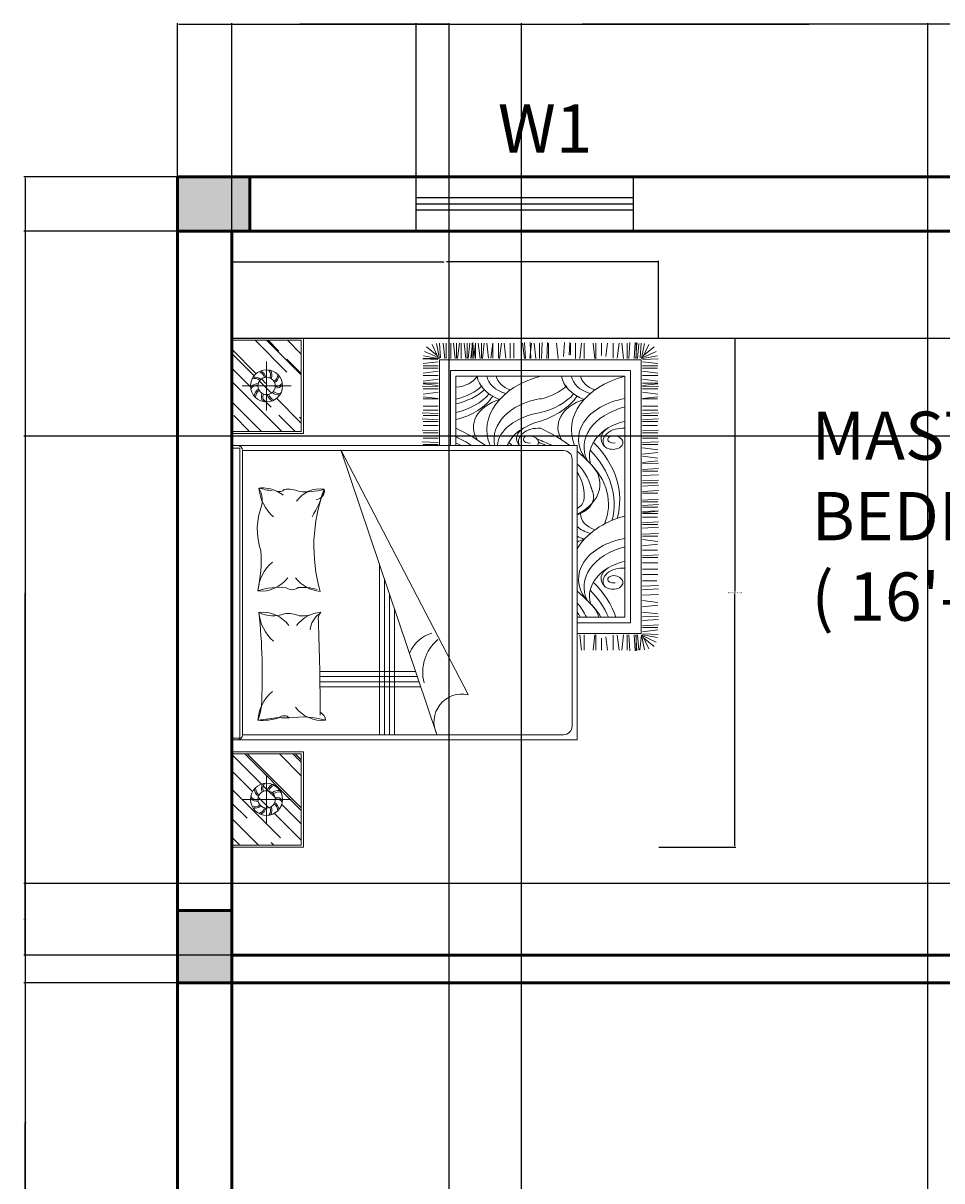
# Model space of a CAD drawing. Units: inches. Extents: x -1517 to -668, y -425 to 52.
# Tile 4 of 13: x -1517 to -1365, y -140 to 52. Entities that reach past the tile are written whole.
import ezdxf

# ---------------------------------------------------------------- set-up
doc = ezdxf.new("R2010")
doc.units = ezdxf.units.IN
doc.header["$MEASUREMENT"] = 0
for name, color, linetype, lineweight in [('A-ANNO-DIMS', 2, 'Continuous', 18), ('A-ANNO-TEXT', 7, 'Continuous', 18), ('A-AREA-IDEN', 7, 'Continuous', 25), ('A-COLS-PATT', 252, 'Continuous', 13), ('column', 7, 'Continuous', 50), ('furniture block', 8, 'Continuous', 18), ('walls', 240, 'Continuous', 50), ('windows', 140, 'Continuous', 25)]:
    doc.layers.add(name, color=color, linetype=linetype, lineweight=lineweight)
doc.styles.get("Standard").update_dxf_attribs({"font": 'arial.ttf'})
doc.dimstyles.get("Standard").update_dxf_attribs({"dimtxt": 0.18, "dimasz": 0.18, "dimexe": 0.18, "dimexo": 0.0625, "dimgap": 0.09, "dimtad": 0, "dimtih": 1, "dimtoh": 1, "dimdec": 4, "dimzin": 0, "dimdsep": 46, "dimlunit": 4, "dimtxsty": 'Standard', "dimcen": 0.09, "dimadec": 0, "dimazin": 0, "dimtfac": 1, "dimtdec": 4, "dimtofl": 0, "dimtmove": 0, "dimatfit": 3, "dimfxl": 1, "dimtolj": 1, "dimtzin": 0, "dimarcsym": 0})

# ---------------------------------------------------------------- blocks, each defined once
blk = doc.blocks.new('column')
for p, q in [((0, 9), (0, 0)), ((12, 9), (0, 9)), ((12, 0), (12, 9)), ((0, 0), (12, 0))]:
    blk.add_line(p, q)
blk = doc.blocks.new('window 3ft')
for p, q in [((9, 36), (0, 36)), ((3.5, 36), (3.5, 0)), ((4.5, 36), (4.5, 0)), ((5.5, 36), (5.5, 0)), ((9, 0), (0, 0))]:
    blk.add_line(p, q)
blk = doc.blocks.new('A$C64B41DC1')
for p, q in [((0, 2.5079), (2.9903, 2.5079)), ((0, 2.0879), (0, 2.5079)), ((0.012, 2.4618), (0.0581, 2.5079)), ((0.012, 2.3515), (0.1684, 2.5079)), ((0.012, 2.0999), (0.012, 2.5079)), ((0.0543, 2.2213), (0.3409, 2.5079)), ((0.1689, 2.4179), (0.2589, 2.5079)), ((0.3265, 2.386), (0.4484, 2.5079)), ((0.3699, 2.3332), (0.5445, 2.5079)), ((0.548, 2.5079), (0.548, 2.0999)), ((0.56, 2.5079), (0.56, 2.0879)), ((0.6301, 2.5079), (0.6301, 0.4779)), ((0.6401, 2.461), (0.6401, 2.5079)), ((0.6401, 2.5079), (2.344, 2.5079)), ((2.344, 2.461), (0.6401, 2.461)), ((2.344, 2.5079), (2.3601, 2.5079)), ((2.344, 2.5079), (2.344, 2.461)), ((2.3601, 2.5079), (2.3601, 2.4761)), ((2.3601, 0.4779), (2.3601, 2.5079)), ((2.4303, 2.5079), (2.4303, 2.0879)), ((2.4423, 2.5079), (2.4423, 2.0999)), ((2.4423, 2.3333), (2.6169, 2.5079)), ((2.4423, 2.2145), (2.7357, 2.5079)), ((2.4423, 2.404), (2.5354, 2.4971)), ((2.705, 2.398), (2.8149, 2.5079)), ((2.7691, 2.3772), (2.8998, 2.5079)), ((2.7819, 2.3646), (2.9252, 2.5079)), ((2.9783, 2.0999), (2.9783, 2.5079)), ((2.9903, 2.0879), (2.9903, 2.5079)), ((0.2157, 2.0999), (0.548, 2.4322)), ((0.2299, 2.0999), (0.548, 2.418)), ((0.2804, 2.1597), (0.2804, 2.4481)), ((0.6601, 2.4461), (1.4951, 2.4461)), ((0.6601, 2.4461), (0.6601, 0.5579)), ((1.4951, 2.4461), (0.6697, 2.4461)), ((2.3301, 2.4461), (1.4951, 2.4461)), ((2.3301, 0.5579), (2.3301, 2.4461)), ((2.7099, 2.1597), (2.7099, 2.4481)), ((0.2311, 2.2906), (0.2937, 2.3532)), ((0.3405, 2.3039), (0.3605, 2.3238)), ((2.6158, 2.3088), (2.6313, 2.3243)), ((2.6674, 2.2756), (2.7382, 2.3464)), ((2.7249, 2.3076), (2.7512, 2.3339)), ((2.7914, 2.1846), (2.9783, 2.3715)), ((0.012, 2.261), (0.0275, 2.2765)), ((0.0404, 2.0999), (0.1982, 2.2578)), ((0.1362, 2.3039), (0.4246, 2.3039)), ((0.2905, 2.2539), (0.3304, 2.2938)), ((2.8541, 2.3039), (2.5657, 2.3039)), ((2.5849, 2.2779), (2.6158, 2.3088)), ((2.7746, 2.0999), (2.9783, 2.3036)), ((2.9144, 2.2312), (2.9783, 2.2951)), ((0.1365, 2.0999), (0.251, 2.2144)), ((0.4194, 2.0999), (0.548, 2.2285)), ((2.4423, 2.1353), (2.5382, 2.2312)), ((2.4918, 2.0999), (2.6366, 2.2447)), ((2.7831, 2.0999), (2.8678, 2.1846)), ((2.8962, 2.0999), (2.9783, 2.182)), ((0.4986, 2.0999), (0.548, 2.1493)), ((0.5127, 2.0999), (0.548, 2.1352)), ((2.5172, 2.0999), (2.5269, 2.1096)), ((0.56, 2.0879), (0, 2.0879)), ((0.548, 2.0999), (0.012, 2.0999)), ((2.4303, 2.0879), (2.9903, 2.0879)), ((2.4423, 2.0999), (2.9783, 2.0999)), ((0.9415, 1.9902), (0.9415, 1.3975)), ((0.9715, 1.9906), (0.9715, 1.4076)), ((1.0015, 1.991), (1.0015, 1.4177)), ((1.0315, 1.9916), (1.0315, 1.4279)), ((2.3349, 1.8678), (0.6613, 1.3029)), ((0.8956, 1.1191), (2.3349, 1.8678)), ((1.6636, 1.6412), (0.6601, 1.6412)), ((1.5748, 1.6112), (0.6601, 1.6112)), ((2.3665, 1.295), (2.3665, 1.3839)), ((2.377, 1.295), (2.3822, 1.3891)), ((2.4032, 1.295), (2.4032, 1.3839)), ((2.4346, 1.295), (2.4346, 1.3839)), ((2.4451, 1.295), (2.4503, 1.3891)), ((2.4774, 1.2957), (2.4774, 1.3837)), ((2.5, 1.295), (2.5, 1.3839)), ((2.5105, 1.295), (2.5157, 1.3891)), ((2.5367, 1.295), (2.5367, 1.3839)), ((2.5471, 1.295), (2.5524, 1.3891)), ((2.5681, 1.295), (2.5681, 1.3839)), ((2.5918, 1.295), (2.5918, 1.3839)), ((2.6346, 1.2957), (2.6346, 1.3837)), ((2.6362, 1.2957), (2.6467, 1.3839)), ((2.6729, 1.295), (2.6624, 1.3839)), ((2.6938, 1.295), (2.6938, 1.3839)), ((2.7043, 1.295), (2.7095, 1.3891)), ((2.7127, 1.2957), (2.7232, 1.3839)), ((2.7253, 1.295), (2.7253, 1.3839)), ((2.7494, 1.295), (2.7389, 1.3839)), ((2.7718, 1.295), (2.7718, 1.3839)), ((2.7959, 1.295), (2.7854, 1.3839)), ((2.8146, 1.2957), (2.8146, 1.3837)), ((2.8146, 1.2957), (2.8146, 1.3837)), ((2.8282, 1.295), (2.8282, 1.3839)), ((2.8282, 1.295), (2.8282, 1.3839)), ((2.8523, 1.295), (2.8418, 1.3839)), ((2.8523, 1.295), (2.8418, 1.3839)), ((2.8653, 1.2966), (2.8688, 1.3861)), ((2.8711, 1.2957), (2.8711, 1.3837)), ((2.8711, 1.2957), (2.8875, 1.3822)), ((2.8765, 1.2958), (2.9132, 1.3758)), ((2.8893, 1.3011), (2.9394, 1.3636)), ((2.8713, 1.2927), (2.954, 1.3315)), ((2.8717, 1.2884), (2.9588, 1.3058)), ((2.3601, 1.2873), (2.8639, 1.2873)), ((2.8639, 1.2873), (2.8639, 0.1018)), ((2.8716, 1.2565), (2.9605, 1.2669)), ((2.8723, 1.2489), (2.9603, 1.2489)), ((2.8744, 1.2817), (2.9603, 1.2869)), ((2.3601, 1.2233), (2.7999, 1.2233)), ((2.3601, 1.1913), (2.7679, 1.1912)), ((2.7679, 1.1912), (2.7679, 0.1978)), ((2.7999, 1.2233), (2.7999, 0.1658)), ((2.8716, 1.2212), (2.9605, 1.2212)), ((2.8716, 1.1947), (2.9605, 1.2052)), ((2.8716, 1.181), (2.9605, 1.1705)), ((2.8716, 1.1595), (2.9605, 1.1595)), ((2.8723, 1.1872), (2.9603, 1.1872)), ((2.8716, 1.133), (2.9605, 1.1435)), ((2.8716, 1.1193), (2.9605, 1.1088)), ((2.8716, 1.1035), (2.9605, 1.093)), ((2.8716, 1.0965), (2.9605, 1.0965)), ((2.8716, 1.086), (2.9657, 1.0913)), ((2.8723, 1.1255), (2.9603, 1.1255)), ((2.8716, 1.0756), (2.9605, 1.0756)), ((2.8716, 1.0491), (2.9605, 1.0596)), ((2.8716, 1.0354), (2.9605, 1.0249)), ((2.8723, 1.0858), (2.9605, 1.0753)), ((2.8723, 1.0416), (2.9603, 1.0416)), ((2.8723, 0.9987), (2.9605, 1.0092)), ((2.8723, 0.985), (2.9605, 0.9745)), ((2.8723, 0.9735), (2.9603, 0.9735)), ((2.8716, 0.9346), (2.9605, 0.9241)), ((2.8723, 0.9408), (2.9603, 0.9408)), ((2.8723, 0.8979), (2.9605, 0.9084)), ((2.8723, 0.8726), (2.9603, 0.8726)), ((2.8723, 0.8505), (2.9603, 0.8505)), ((2.8716, 0.7885), (2.9605, 0.799)), ((2.8716, 0.7818), (2.9657, 0.787)), ((2.8716, 0.7503), (2.9657, 0.7556)), ((2.8723, 0.7571), (2.9605, 0.7466)), ((2.8716, 0.7204), (2.9605, 0.7309)), ((2.8716, 0.6995), (2.9605, 0.6995)), ((2.8716, 0.689), (2.9657, 0.6838)), ((2.8716, 0.6576), (2.9657, 0.6523)), ((2.8716, 0.6471), (2.9605, 0.6471)), ((2.8716, 0.5903), (2.9605, 0.6007)), ((2.882, 0.5582), (2.9657, 0.5536)), ((0.6301, 0.4779), (2.3601, 0.4779)), ((0.7101, 0.5079), (2.2801, 0.5079)), ((1.2542, 0.1018), (1.2542, 0.4779)), ((1.3182, 0.1658), (1.3182, 0.4779)), ((1.3502, 0.1978), (1.3502, 0.4779)), ((2.8716, 0.4877), (2.9603, 0.4877)), ((2.8909, 0.5263), (2.9657, 0.5222)), ((2.8928, 0.5169), (2.9605, 0.5169)), ((1.2465, 0.4625), (1.1576, 0.452)), ((1.2465, 0.4365), (1.1577, 0.4365)), ((2.8716, 0.4625), (2.9605, 0.452)), ((2.8716, 0.4365), (2.9603, 0.4365)), ((1.2465, 0.3746), (1.1576, 0.3851)), ((1.2465, 0.3684), (1.1577, 0.3684)), ((2.8716, 0.3746), (2.9605, 0.3851)), ((2.8716, 0.3684), (2.9603, 0.3684)), ((1.2355, 0.3092), (1.1576, 0.3)), ((1.2285, 0.3357), (1.1577, 0.3357)), ((2.8826, 0.3092), (2.9605, 0.3)), ((2.8896, 0.3357), (2.9603, 0.3357)), ((1.2457, 0.2423), (1.1576, 0.2319)), ((1.2465, 0.2057), (1.1576, 0.2161)), ((1.2457, 0.2676), (1.1577, 0.2676)), ((2.8716, 0.2057), (2.9605, 0.2161)), ((2.8723, 0.2676), (2.9603, 0.2676)), ((2.8723, 0.2423), (2.9605, 0.2319)), ((1.2465, 0.1742), (1.1524, 0.169)), ((1.2465, 0.1428), (1.1524, 0.1376)), ((1.2465, 0.1847), (1.1576, 0.1847)), ((2.7999, 0.1658), (1.3182, 0.1658)), ((2.7679, 0.1978), (1.3502, 0.1978)), ((2.8716, 0.1847), (2.9605, 0.1847)), ((2.8716, 0.1742), (2.9657, 0.169)), ((2.8716, 0.1428), (2.9657, 0.1376)), ((1.2465, 0.1334), (1.1524, 0.1281)), ((1.2465, 0.1323), (1.1576, 0.1323)), ((1.2465, 0.1323), (1.1576, 0.1323)), ((1.2465, 0.1), (1.1576, 0.1105)), ((1.2465, 0.1229), (1.1588, 0.1168)), ((1.2464, 0.1007), (1.1592, 0.0833)), ((1.2468, 0.0964), (1.1641, 0.0576)), ((1.2288, 0.088), (1.1787, 0.0255)), ((1.2415, 0.0933), (1.2049, 0.0133)), ((1.247, 0.0934), (1.2306, 0.0069)), ((1.2527, 0.0925), (1.2493, 0.003)), ((2.8639, 0.1018), (1.2542, 0.1018)), ((1.2658, 0.0941), (1.2762, 0.0052)), ((1.2899, 0.0941), (1.2899, 0.0052)), ((1.2999, 0.0941), (1.3051, 0)), ((1.3313, 0.0941), (1.3365, 0)), ((1.3523, 0.0941), (1.3575, 0)), ((1.3804, 0.0941), (1.3699, 0.0052)), ((1.4119, 0.0934), (1.4223, 0.0052)), ((1.4485, 0.0941), (1.438, 0.0052)), ((1.48, 0.0941), (1.4852, 0)), ((1.5114, 0.0941), (1.5166, 0)), ((1.5323, 0.0941), (1.5376, 0)), ((1.5638, 0.0941), (1.5638, 0.0105)), ((1.6021, 0.0941), (1.6021, 0.0052)), ((1.6336, 0.0941), (1.6336, 0.0052)), ((1.6702, 0.0941), (1.6702, 0.0052)), ((1.7017, 0.0941), (1.7017, 0.0052)), ((1.7122, 0.0941), (1.7174, 0)), ((1.7445, 0.0934), (1.7445, 0.0054)), ((1.7698, 0.0934), (1.7803, 0.0052)), ((1.8065, 0.0941), (1.796, 0.0052)), ((1.8274, 0.0941), (1.8274, 0.0052)), ((1.8379, 0.0941), (1.8431, 0)), ((1.8746, 0.0941), (1.8798, 0)), ((1.8955, 0.0941), (1.8955, 0.0052)), ((1.906, 0.0941), (1.9113, 0)), ((1.9384, 0.0934), (1.9384, 0.0054)), ((1.9609, 0.0941), (1.9609, 0.0052)), ((1.9636, 0.0934), (1.9741, 0.0052)), ((1.9714, 0.0941), (1.9766, 0)), ((1.9976, 0.0941), (1.9976, 0.0052)), ((2.0081, 0.0941), (2.0133, 0)), ((2.029, 0.0941), (2.029, 0.0052)), ((2.0395, 0.0941), (2.0447, 0)), ((2.0797, 0.0941), (2.0797, 0.0052)), ((2.0902, 0.0941), (2.0954, 0)), ((2.1216, 0.0941), (2.1269, 0)), ((2.1412, 0.0941), (2.1412, 0.0052)), ((2.1517, 0.0941), (2.1569, 0)), ((2.1831, 0.0941), (2.1884, 0)), ((2.2093, 0.0941), (2.2093, 0.0052)), ((2.2198, 0.0941), (2.225, 0)), ((2.2512, 0.0941), (2.2565, 0)), ((2.2603, 0.0934), (2.2707, 0.0052)), ((2.2969, 0.0941), (2.2864, 0.0052)), ((2.3089, 0.0934), (2.3193, 0.0052)), ((2.3455, 0.0941), (2.3351, 0.0052)), ((2.3665, 0.0941), (2.3665, 0.0052)), ((2.377, 0.0941), (2.3822, 0)), ((2.4032, 0.0941), (2.4032, 0.0052)), ((2.4346, 0.0941), (2.4346, 0.0052)), ((2.4451, 0.0941), (2.4503, 0)), ((2.4774, 0.0934), (2.4774, 0.0054)), ((2.5, 0.0941), (2.5, 0.0052)), ((2.5105, 0.0941), (2.5157, 0)), ((2.5367, 0.0941), (2.5367, 0.0052)), ((2.5471, 0.0941), (2.5524, 0)), ((2.5681, 0.0941), (2.5681, 0.0052)), ((2.5918, 0.0941), (2.5918, 0.0052)), ((2.6346, 0.0934), (2.6346, 0.0054)), ((2.6362, 0.0934), (2.6467, 0.0052)), ((2.6729, 0.0941), (2.6624, 0.0052)), ((2.6938, 0.0941), (2.6938, 0.0052)), ((2.7043, 0.0941), (2.7095, 0)), ((2.7127, 0.0934), (2.7232, 0.0052)), ((2.7253, 0.0941), (2.7253, 0.0052)), ((2.7494, 0.0941), (2.7389, 0.0052)), ((2.7718, 0.0941), (2.7718, 0.0052)), ((2.7959, 0.0941), (2.7854, 0.0052)), ((2.8146, 0.0934), (2.8146, 0.0054)), ((2.8282, 0.0941), (2.8282, 0.0052)), ((2.8523, 0.0941), (2.8418, 0.0052)), ((2.8653, 0.0925), (2.8688, 0.003)), ((2.8711, 0.0934), (2.8875, 0.0069)), ((2.8713, 0.0964), (2.954, 0.0576)), ((2.8716, 0.1334), (2.9657, 0.1281)), ((2.8716, 0.1323), (2.9605, 0.1323)), ((2.8716, 0.1229), (2.9593, 0.1168)), ((2.8717, 0.1007), (2.9588, 0.0833)), ((2.8744, 0.1074), (2.9603, 0.1022)), ((2.8765, 0.0933), (2.9132, 0.0133)), ((2.8893, 0.088), (2.9394, 0.0255))]:
    blk.add_line(p, q)
at = {"ltscale": 10}
for p, q in [((1.4859, 1.5812), (0.6601, 1.5812)), ((1.397, 1.5512), (0.6601, 1.5512))]:
    blk.add_line(p, q, dxfattribs=at)
for centre, radius in [((0.2804, 2.3039), 0.0942), ((2.7099, 2.3039), 0.0942), ((0.2804, 2.3039), 0.051), ((2.7099, 2.3039), 0.051)]:
    blk.add_circle(centre, radius)
for centre, radius, start, end in [((0.6601, 2.4761), 0.03, 180, 270), ((2.3301, 2.4761), 0.03, 270, 0), ((0.2887, 2.3745), 0.0605, 172.17003, 218.48975), ((0.2828, 2.3731), 0.0462, 160.30017, 220.53802), ((0.3286, 2.3561), 0.0605, 136.17003, 182.48975), ((0.3231, 2.3585), 0.0462, 124.30017, 184.53802), ((2.6672, 2.3585), 0.0462, 355.46198, 55.69983), ((2.6617, 2.3561), 0.0605, 357.51025, 43.82997), ((2.7075, 2.3731), 0.0462, 319.46198, 19.69983), ((2.7016, 2.3745), 0.0605, 321.51025, 7.82997), ((0.2457, 2.3659), 0.0605, 208.17003, 254.48975), ((0.2417, 2.3614), 0.0462, 196.30017, 256.53802), ((0.3501, 2.3178), 0.0605, 100.17003, 146.48975), ((0.347, 2.323), 0.0462, 88.30017, 148.53802), ((0.3449, 2.2742), 0.0605, 64.17003, 110.48975), ((0.3455, 2.2802), 0.0462, 52.30017, 112.53802), ((1.0526, 2.3302), 0.3085, 175.30484, 198.69419), ((-0.8702, 2.0941), 1.6364, 4.80985, 9.18918), ((0.8579, 2.6278), 0.2948, 247.51785, 264.26696), ((0.728, 2.111), 0.245, 40.4189, 85.9871), ((1.0164, 5.7096), 3.3803, 266.81337, 276.16021), ((1.3963, 2.1044), 0.245, 94.0129, 139.5811), ((1.1858, 2.3288), 0.1943, 306.5711, 5.88998), ((1.5348, 2.2652), 0.1767, 151.77364, 201.69827), ((1.6986, 2.3355), 0.1943, 174.11002, 233.4289), ((1.1481, 2.2311), 0.3783, 353.49469, 19.18669), ((1.6871, 3.192), 0.8561, 257.74383, 273.62843), ((1.4882, 2.111), 0.245, 40.4189, 85.9871), ((1.8674, 1.9709), 0.3878, 68.20259, 108.9817), ((2.1269, 2.1044), 0.245, 94.0129, 139.5811), ((2.0342, 2.4856), 0.1563, 261.59582, 298.90918), ((1.9165, 2.3288), 0.1943, 333.73715, 5.88998), ((2.6058, 2.2028), 0.517, 163.60457, 172.3273), ((2.6448, 2.2802), 0.0462, 67.46198, 127.69983), ((2.6454, 2.2742), 0.0605, 69.51025, 115.82997), ((2.6433, 2.323), 0.0462, 31.46198, 91.69983), ((2.6402, 2.3178), 0.0605, 33.51025, 79.82997), ((2.7486, 2.3614), 0.0462, 283.46198, 343.69983), ((2.7446, 2.3659), 0.0605, 285.51025, 331.82997), ((0.2153, 2.3276), 0.0462, 232.30017, 292.53802), ((0.2158, 2.3336), 0.0605, 244.17003, 290.48975), ((0.2138, 2.2848), 0.0462, 268.30017, 328.53802), ((0.2107, 2.29), 0.0605, 280.17003, 326.48975), ((0.2377, 2.2493), 0.0462, 304.30017, 4.53802), ((0.2322, 2.2517), 0.0605, 316.17003, 2.48975), ((0.2779, 2.2347), 0.0462, 340.30017, 40.53802), ((0.272, 2.2333), 0.0605, 352.17003, 38.48975), ((0.3191, 2.2464), 0.0462, 16.30017, 76.53802), ((0.3151, 2.2419), 0.0605, 28.17003, 74.48975), ((2.6752, 2.2419), 0.0605, 105.51025, 151.82997), ((2.6712, 2.2464), 0.0462, 103.46198, 163.69983), ((2.7182, 2.2333), 0.0605, 141.51025, 187.82997), ((2.7123, 2.2347), 0.0462, 139.46198, 199.69983), ((2.7581, 2.2517), 0.0605, 177.51025, 223.82997), ((2.7526, 2.2493), 0.0462, 175.46198, 235.69983), ((2.7796, 2.29), 0.0605, 213.51025, 259.82997), ((2.7765, 2.2848), 0.0462, 211.46198, 271.69983), ((2.7744, 2.3336), 0.0605, 249.51025, 295.82997), ((2.775, 2.3276), 0.0462, 247.46198, 307.69983), ((0.7274, 2.2013), 0.0446, 314.4736, 42.17134), ((-1.6008, 2.277), 2.3618, 357.39054, 358.88764), ((1.204, 2.1778), 0.1681, 337.01697, 7.53676), ((1.5671, 2.1546), 0.0547, 142.08329, 220.902), ((1.9165, 2.3288), 0.1943, 320.94042, 333.73715), ((2.1347, 2.2313), 0.0459, 165.35061, 223.26844), ((1.9346, 2.1778), 0.1681, 337.01697, 7.53676), ((0.9385, 1.978), 0.1943, 126.5711, 185.88998), ((0.2688, 2.0945), 0.4956, 344.0243, 8.70709), ((1.1858, 1.9714), 0.1943, 4.31813, 53.4289), ((1.5415, 2.0969), 0.1834, 175.22328, 196.23004), ((1.7059, 1.9714), 0.204, 127.11975, 175.09005), ((1.1965, 2.0983), 0.3299, 343.79543, 3.55541), ((1.9394, 1.991), 0.1651, 351.26213, 55.75721), ((2.4617, 2.0719), 0.3745, 173.82958, 196.4356), ((1.2687, 1.9248), 0.1223, 33.62799, 86.47438), ((0.7417, 2.0149), 0.057, 273.47085, 328.54118), ((0.7246, 18.8439), 16.8552, 270.17399, 272.05214), ((1.3401, 1.9404), 0.0603, 49.09906, 101.37023), ((1.7676, 1.0629), 0.9631, 69.65065, 105.96307), ((2.2748, 2.5795), 0.6373, 238.34989, 254.31375), ((2.0911, 2.0123), 0.0478, 179.77267, 283.80184), ((0.728, 2.2025), 0.245, 274.0129, 278.34166), ((1.0747, 1.2871), 0.1871, 14.1863, 69.12121), ((1.0274, 1.1334), 0.2527, 40.62904, 104.37123), ((0.7347, 1.1553), 0.1649, 347.31088, 116.44537), ((0.7101, 0.5579), 0.05, 180, 270), ((2.2801, 0.5579), 0.05, 270, 0)]:
    blk.add_arc(centre, radius, start, end)
for centre, major_axis, ratio, start_param, end_param in [((1.9938, 1.6262), (0, -0.7531), 0.68, 0.797284, 0.954936), ((2.0643, 1.466), (0, -0.5322), 0.68, 7.239912, 7.311536), ((1.9052, 1.7397), (0, -0.9842), 0.68, 0.74745, 0.979724), ((2.7455, 1.3081), (0, 0.3614), 0.68, 1.900046, 2.742661), ((2.7868, 1.3081), (0, 0.3614), 0.68, 1.900046, 2.614747), ((2.8372, 1.3081), (0, 0.3614), 0.68, 1.900046, 2.479658), ((2.8607, 1.3211), (0, 0.3614), 0.68, 1.938265, 2.479658), ((2.8057, 1.2079), (0, -0.1524), 0.68, 4.821745, 5.895886), ((2.4665, 0.8216), (0, -0.2664), 0.68, 2.006169, 3.565187), ((2.4513, 0.5069), (0, 0.502), 0.68, 5.095327, 6.553458), ((2.7862, 0.8069), (0, -0.2615), 0.68, 3.244645, 4.205018), ((2.396, 0.6032), (0, 0.3641), 0.68, -1.3172, 0.145284), ((2.7784, 0.8289), (0, -0.1802), 0.68, 3.227058, 4.318474), ((2.7821, 0.7971), (0, -0.1589), 0.68, 3.272942, 4.229533), ((2.3507, 0.5642), (0.0073, 0.3819), 0.56205, -1.21172, -0.009991), ((2.2964, 0.5771), (0, -0.3263), 0.68, 1.938944, 2.850232), ((2.0403, 1.6015), (0, -0.8763), 0.68, 6.849801, 6.887077), ((2.4005, 0.7132), (0, -0.1214), 0.68, 2.284368, 3.652258), ((2.3834, 0.7081), (0, 0.1147), 0.68, 4.593909, 6.585576), ((2.3774, 0.7653), (0, -0.0593), 0.68, 5.841311, 7.755362), ((2.3961, 0.7628), (0, -0.0317), 0.68, 1.462497, 5.046281), ((1.9938, 1.1295), (-0.0678, 0.7439), 0.610498, 3.917146, 4.063997), ((2.0643, 0.9693), (0, -0.5322), 0.68, 7.239912, 7.336618), ((1.9052, 1.243), (0, -0.9842), 0.68, 0.74745, 0.979724), ((2.7455, 0.8114), (-0.0599, 0.3735), 0.695517, 1.775813, 2.548612), ((2.7868, 0.8114), (0, 0.3614), 0.68, 1.900046, 2.614747), ((2.8607, 0.8243), (0, 0.3614), 0.68, 1.938265, 2.479658), ((2.4665, 0.3249), (0, -0.2664), 0.68, 2.006169, 3.565187), ((2.4513, 0.0102), (0, 0.502), 0.68, 5.095327, 6.553458), ((2.7862, 0.3102), (0, -0.2615), 0.68, 3.244645, 4.205018), ((1.242, 0.9693), (0, -0.5322), 0.68, 6.586764, 6.677612), ((1.1714, 1.1295), (-0.1157, 0.7241), 0.59432, 3.291697, 3.50733), ((1.0828, 1.243), (0, -0.9842), 0.68, 0.565948, 0.680366), ((1.5283, 0.0674), (0, -0.3703), 0.68, 1.930561, 3.464283), ((1.5736, 0.1065), (0, 0.3641), 0.68, -1.3172, 0.476403), ((1.6289, 0.0102), (0, 0.502), 0.68, 6.655152, 6.661293), ((1.6289, 0.0102), (0, 0.502), 0.68, 5.095327, 5.911219), ((1.6442, 0.3249), (0, -0.2664), 0.68, 2.006169, 2.182797), ((1.9638, 0.3102), (0, -0.2615), 0.68, 4.015924, 4.205018), ((1.956, 0.3322), (0, -0.1802), 0.68, 3.770744, 4.318474), ((2.0606, 0.5616), (0, -0.1803), 0.68, 5.194792, 5.929328), ((2.0606, 0.5616), (0, -0.1803), 0.68, 5.194792, 6.723255), ((2.1315, 0.6603), (0, -0.3155), 0.68, 5.328638, 6.949396), ((2.0549, 0.5656), (0, -0.1303), 0.68, 5.450951, 6.054641), ((2.0643, 0.9693), (0, -0.5322), 0.68, 6.20013, 6.677612), ((1.9938, 1.1295), (-0.0678, 0.7439), 0.610498, 3.199135, 3.592282), ((1.9052, 1.243), (0, -0.9842), 0.68, 0.565948, 0.680366), ((2.3507, 0.0674), (0, -0.3703), 0.68, 1.930561, 3.464283), ((2.396, 0.1065), (0, 0.3641), 0.68, -1.3172, 0.476403), ((2.4513, 0.0102), (0, 0.502), 0.68, 6.655152, 6.661293), ((2.7784, 0.3322), (0, -0.1802), 0.68, 3.227058, 4.318474), ((1.1933, 0.9181), (0, -0.624), 0.68, 0.378672, 0.625379), ((1.3091, 0.6603), (0, -0.3155), 0.68, 6.475719, 6.949396), ((1.474, 0.0804), (0, -0.3263), 0.68, 1.938944, 3.339184), ((1.9597, 0.3004), (0, -0.1589), 0.68, 3.14258, 4.229533), ((2.0157, 0.9181), (0, -0.624), 0.68, -0.280078, 0.625379), ((2.2964, 0.0804), (0, -0.3263), 0.68, 1.938944, 3.339184), ((2.7821, 0.3004), (0, -0.1589), 0.68, 3.272942, 4.229533), ((1.1911, 1.1066), (0, 0.8458), 0.68, 3.421828, 3.728616), ((1.2179, 1.1047), (0, -0.8763), 0.68, 6.507006, 6.887077), ((1.5781, 0.2165), (0, -0.1214), 0.68, 2.284368, 3.726131), ((2.0135, 1.1066), (0, 0.8458), 0.68, 2.978727, 3.728616), ((2.0403, 1.1047), (0, -0.8763), 0.68, 6.099302, 6.887077), ((2.4005, 0.2165), (0, -0.1214), 0.68, 2.284368, 3.726131), ((1.555, 0.2685), (0, -0.0593), 0.68, 3.732151, 7.755362), ((1.561, 0.2114), (0, 0.1147), 0.68, 4.593909, 6.647252), ((1.5737, 0.2661), (0, -0.0317), 0.68, 1.462497, 5.046281), ((2.3774, 0.2685), (0, -0.0593), 0.68, 3.732151, 7.755362), ((2.3834, 0.2114), (0, 0.1147), 0.68, 4.593909, 6.647252), ((2.3961, 0.2661), (0, -0.0317), 0.68, 1.462497, 5.046281)]:
    blk.add_ellipse(centre, major_axis=major_axis, ratio=ratio, start_param=start_param, end_param=end_param)
blk = doc.blocks.new('*D34')
at = {"layer": 'A-ANNO-DIMS', "color": 0, "lineweight": -2, "transparency": 16777216}
for p, q in [((-1411.71, -0.11), (-1398.94, -0.11)), ((-1399.12, -0.29), (-1399.12, -42.1)), ((-1399.12, -84.27), (-1399.12, -42.47)), ((-1411.71, -84.45), (-1398.94, -84.45))]:
    blk.add_line(p, q, dxfattribs=at)
at = {"layer": 'A-ANNO-DIMS', "color": 0, "transparency": 16777216}
for points in [[(-1399.15, -0.29), (-1399.09, -0.29), (-1399.12, -0.11)], [(-1399.15, -84.27), (-1399.09, -84.27), (-1399.12, -84.45)]]:
    blk.add_solid(points, dxfattribs=at)
at = {"layer": 'Defpoints', "color": 0, "transparency": 16777216}
for p in [(-1411.77, -0.11), (-1399.12, -0.11), (-1411.77, -84.45)]:
    blk.add_point(p, dxfattribs=at)
at = {"layer": 'A-ANNO-DIMS', "color": 0, "transparency": 16777216, "insert": (-1399.12, -42.28), "char_height": 0.18, "attachment_point": 5}
blk.add_mtext('\\A1;MASTER BED SET 84', dxfattribs=at)
blk = doc.blocks.new('*D35')
at = {"layer": 'A-ANNO-DIMS', "color": 0, "lineweight": -2, "transparency": 16777216}
for p, q in [((-1482.5, -0.05), (-1482.5, 12.72)), ((-1482.32, 12.54), (-1447.34, 12.54)), ((-1411.95, 12.54), (-1446.94, 12.54)), ((-1411.77, -0.05), (-1411.77, 12.72))]:
    blk.add_line(p, q, dxfattribs=at)
at = {"layer": 'A-ANNO-DIMS', "color": 0, "transparency": 16777216}
for points in [[(-1482.32, 12.57), (-1482.32, 12.51), (-1482.5, 12.54)], [(-1411.95, 12.57), (-1411.95, 12.51), (-1411.77, 12.54)]]:
    blk.add_solid(points, dxfattribs=at)
at = {"layer": 'Defpoints', "color": 0, "transparency": 16777216}
for p in [(-1482.5, 12.54), (-1482.5, -0.11), (-1411.77, -0.11)]:
    blk.add_point(p, dxfattribs=at)
at = {"layer": 'A-ANNO-DIMS', "color": 0, "transparency": 16777216, "insert": (-1447.14, 12.54), "char_height": 0.18, "attachment_point": 5}
blk.add_mtext('\\A1;71', dxfattribs=at)
blk = doc.blocks.new('*D45')
at = {"layer": 'A-ANNO-DIMS', "color": 0, "lineweight": -2, "transparency": 16777216}
for p, q in [((-1491.57, 26.63), (-1516.98, 26.63)), ((-1516.8, 26.45), (-1516.8, -162.19)), ((-1516.8, -351.19), (-1516.8, -162.55)), ((-1491.57, -351.37), (-1516.98, -351.37))]:
    blk.add_line(p, q, dxfattribs=at)
at = {"layer": 'A-ANNO-DIMS', "color": 0, "transparency": 16777216}
for points in [[(-1516.83, 26.45), (-1516.77, 26.45), (-1516.8, 26.63)], [(-1516.83, -351.19), (-1516.77, -351.19), (-1516.8, -351.37)]]:
    blk.add_solid(points, dxfattribs=at)
at = {"layer": 'Defpoints', "color": 0, "transparency": 16777216}
for p in [(-1491.5, 26.63), (-1516.8, -351.37), (-1491.5, -351.37)]:
    blk.add_point(p, dxfattribs=at)
at = {"layer": 'A-ANNO-DIMS', "color": 0, "transparency": 16777216, "insert": (-1516.8, -162.37), "char_height": 0.18, "attachment_point": 5}
blk.add_mtext('\\A1;378', dxfattribs=at)
blk = doc.blocks.new('*D47')
at = {"layer": 'A-ANNO-DIMS', "color": 0, "lineweight": -2, "transparency": 16777216}
for p, q in [((-1482.5, -102.31), (-1482.5, 52.11)), ((-1482.32, 51.93), (-1386.78, 51.93)), ((-1290.68, 51.93), (-1386.22, 51.93)), ((-1290.5, -102.31), (-1290.5, 52.11))]:
    blk.add_line(p, q, dxfattribs=at)
at = {"layer": 'A-ANNO-DIMS', "color": 0, "transparency": 16777216}
for points in [[(-1482.32, 51.96), (-1482.32, 51.9), (-1482.5, 51.93)], [(-1290.68, 51.96), (-1290.68, 51.9), (-1290.5, 51.93)]]:
    blk.add_solid(points, dxfattribs=at)
at = {"layer": 'Defpoints', "color": 0, "transparency": 16777216}
for p in [(-1290.5, 51.93), (-1482.5, -102.37), (-1290.5, -102.37)]:
    blk.add_point(p, dxfattribs=at)
at = {"layer": 'A-ANNO-DIMS', "color": 0, "transparency": 16777216, "insert": (-1386.5, 51.93), "char_height": 0.18, "attachment_point": 5}
blk.add_mtext('\\A1;192', dxfattribs=at)
blk = doc.blocks.new('*D51')
at = {"layer": 'A-ANNO-DIMS', "color": 0, "lineweight": -2, "transparency": 16777216}
for p, q in [((-1482.5, -273.31), (-1482.5, 52.11)), ((-1482.32, 51.93), (-1425.19, 51.93)), ((-1367.28, 51.93), (-1424.42, 51.93)), ((-1367.1, -273.31), (-1367.1, 52.11))]:
    blk.add_line(p, q, dxfattribs=at)
at = {"layer": 'A-ANNO-DIMS', "color": 0, "transparency": 16777216}
for points in [[(-1482.32, 51.96), (-1482.32, 51.9), (-1482.5, 51.93)], [(-1367.28, 51.96), (-1367.28, 51.9), (-1367.1, 51.93)]]:
    blk.add_solid(points, dxfattribs=at)
at = {"layer": 'Defpoints', "color": 0, "transparency": 16777216}
for p in [(-1367.1, 51.93), (-1482.5, -273.37), (-1367.1, -273.37)]:
    blk.add_point(p, dxfattribs=at)
at = {"layer": 'A-ANNO-DIMS', "color": 0, "transparency": 16777216, "insert": (-1424.8, 51.93), "char_height": 0.18, "attachment_point": 5}
blk.add_mtext('\\A1;115.4', dxfattribs=at)
blk = doc.blocks.new('*D54')
at = {"layer": 'A-ANNO-DIMS', "color": 0, "lineweight": -2, "transparency": 16777216}
for p, q in [((-1482.57, 17.63), (-1516.98, 17.63)), ((-1516.8, 17.45), (-1516.8, -42.19)), ((-1516.8, -102.19), (-1516.8, -42.55)), ((-1482.57, -102.37), (-1516.98, -102.37))]:
    blk.add_line(p, q, dxfattribs=at)
at = {"layer": 'A-ANNO-DIMS', "color": 0, "transparency": 16777216}
for points in [[(-1516.83, 17.45), (-1516.77, 17.45), (-1516.8, 17.63)], [(-1516.83, -102.19), (-1516.77, -102.19), (-1516.8, -102.37)]]:
    blk.add_solid(points, dxfattribs=at)
at = {"layer": 'Defpoints', "color": 0, "transparency": 16777216}
for p in [(-1482.5, 17.63), (-1516.8, -102.37), (-1482.5, -102.37)]:
    blk.add_point(p, dxfattribs=at)
at = {"layer": 'A-ANNO-DIMS', "color": 0, "transparency": 16777216, "insert": (-1516.8, -42.37), "char_height": 0.18, "attachment_point": 5}
blk.add_mtext('\\A1;120', dxfattribs=at)
blk = doc.blocks.new('*D55')
at = {"layer": 'A-ANNO-DIMS', "color": 0, "lineweight": -2, "transparency": 16777216}
for p, q in [((-1482.57, -106.97), (-1516.98, -106.97)), ((-1516.8, -107.15), (-1516.8, -129.99)), ((-1516.8, -153.19), (-1516.8, -130.35)), ((-1482.57, -153.37), (-1516.98, -153.37))]:
    blk.add_line(p, q, dxfattribs=at)
at = {"layer": 'A-ANNO-DIMS', "color": 0, "transparency": 16777216}
for points in [[(-1516.83, -107.15), (-1516.77, -107.15), (-1516.8, -106.97)], [(-1516.83, -153.19), (-1516.77, -153.19), (-1516.8, -153.37)]]:
    blk.add_solid(points, dxfattribs=at)
at = {"layer": 'Defpoints', "color": 0, "transparency": 16777216}
for p in [(-1482.5, -106.97), (-1516.8, -153.37), (-1482.5, -153.37)]:
    blk.add_point(p, dxfattribs=at)
at = {"layer": 'A-ANNO-DIMS', "color": 0, "transparency": 16777216, "insert": (-1516.8, -130.17), "char_height": 0.18, "attachment_point": 5}
blk.add_mtext('\\A1;46.4', dxfattribs=at)
blk = doc.blocks.new('*D59')
at = {"layer": 'A-ANNO-DIMS', "color": 0, "lineweight": -2, "transparency": 16777216}
for p, q in [((-1491.5, 26.69), (-1491.5, 52.11)), ((-1491.32, 51.93), (-1472.19, 51.93)), ((-1452.13, 51.93), (-1471.26, 51.93)), ((-1451.95, 26.69), (-1451.95, 52.11))]:
    blk.add_line(p, q, dxfattribs=at)
at = {"layer": 'A-ANNO-DIMS', "color": 0, "transparency": 16777216}
for points in [[(-1491.32, 51.96), (-1491.32, 51.9), (-1491.5, 51.93)], [(-1452.13, 51.96), (-1452.13, 51.9), (-1451.95, 51.93)]]:
    blk.add_solid(points, dxfattribs=at)
at = {"layer": 'Defpoints', "color": 0, "transparency": 16777216}
for p in [(-1451.95, 51.93), (-1491.5, 26.63), (-1451.95, 26.63)]:
    blk.add_point(p, dxfattribs=at)
at = {"layer": 'A-ANNO-DIMS', "color": 0, "transparency": 16777216, "insert": (-1471.73, 51.93), "char_height": 0.18, "attachment_point": 5}
blk.add_mtext('\\A1;39.555', dxfattribs=at)
blk = doc.blocks.new('*D63')
at = {"layer": 'A-ANNO-DIMS', "color": 0, "lineweight": -2, "transparency": 16777216}
for p, q in [((-1434.48, -282.31), (-1434.48, 52.11)), ((-1434.3, 51.93), (-1401.19, 51.93)), ((-1367.28, 51.93), (-1400.4, 51.93)), ((-1367.1, -282.31), (-1367.1, 52.11))]:
    blk.add_line(p, q, dxfattribs=at)
at = {"layer": 'A-ANNO-DIMS', "color": 0, "transparency": 16777216}
for points in [[(-1434.3, 51.96), (-1434.3, 51.9), (-1434.48, 51.93)], [(-1367.28, 51.96), (-1367.28, 51.9), (-1367.1, 51.93)]]:
    blk.add_solid(points, dxfattribs=at)
at = {"layer": 'Defpoints', "color": 0, "transparency": 16777216}
for p in [(-1367.1, 51.93), (-1434.48, -282.37), (-1367.1, -282.37)]:
    blk.add_point(p, dxfattribs=at)
at = {"layer": 'A-ANNO-DIMS', "color": 0, "transparency": 16777216, "insert": (-1400.79, 51.93), "char_height": 0.18, "attachment_point": 5}
blk.add_mtext('\\A1;67.38', dxfattribs=at)
blk = doc.blocks.new('*D67')
at = {"layer": 'A-ANNO-DIMS', "color": 0, "lineweight": -2, "transparency": 16777216}
for p, q in [((-1482.5, -157.91), (-1482.5, 52.11)), ((-1482.32, 51.93), (-1464.72, 51.93)), ((-1446.68, 51.93), (-1464.28, 51.93)), ((-1446.5, -157.91), (-1446.5, 52.11))]:
    blk.add_line(p, q, dxfattribs=at)
at = {"layer": 'A-ANNO-DIMS', "color": 0, "transparency": 16777216}
for points in [[(-1482.32, 51.96), (-1482.32, 51.9), (-1482.5, 51.93)], [(-1446.68, 51.96), (-1446.68, 51.9), (-1446.5, 51.93)]]:
    blk.add_solid(points, dxfattribs=at)
at = {"layer": 'Defpoints', "color": 0, "transparency": 16777216}
for p in [(-1446.5, 51.93), (-1482.5, -157.97), (-1446.5, -157.97)]:
    blk.add_point(p, dxfattribs=at)
at = {"layer": 'A-ANNO-DIMS', "color": 0, "transparency": 16777216, "insert": (-1464.5, 51.93), "char_height": 0.18, "attachment_point": 5}
blk.add_mtext('\\A1;36', dxfattribs=at)
blk = doc.blocks.new('*D73')
at = {"layer": 'A-ANNO-DIMS', "color": 0, "lineweight": -2, "transparency": 16777216}
for p, q in [((-1089.37, -16.37), (-1516.98, -16.37)), ((-1516.8, -16.55), (-1516.8, -59.19)), ((-1516.8, -102.19), (-1516.8, -59.55)), ((-1089.37, -102.37), (-1516.98, -102.37))]:
    blk.add_line(p, q, dxfattribs=at)
at = {"layer": 'A-ANNO-DIMS', "color": 0, "transparency": 16777216}
for points in [[(-1516.83, -16.55), (-1516.77, -16.55), (-1516.8, -16.37)], [(-1516.83, -102.19), (-1516.77, -102.19), (-1516.8, -102.37)]]:
    blk.add_solid(points, dxfattribs=at)
at = {"layer": 'Defpoints', "color": 0, "transparency": 16777216}
for p in [(-1089.3, -16.37), (-1516.8, -102.37), (-1089.3, -102.37)]:
    blk.add_point(p, dxfattribs=at)
at = {"layer": 'A-ANNO-DIMS', "color": 0, "transparency": 16777216, "insert": (-1516.8, -59.37), "char_height": 0.18, "attachment_point": 5}
blk.add_mtext('\\A1;86', dxfattribs=at)
blk = doc.blocks.new('*D77')
at = {"layer": 'A-ANNO-DIMS', "color": 0, "lineweight": -2, "transparency": 16777216}
for p, q in [((-1482.44, 17.63), (-980.02, 17.63)), ((-980.2, 17.45), (-980.2, 8.94)), ((-980.2, 0.07), (-980.2, 8.58)), ((-1482.44, -0.11), (-980.02, -0.11))]:
    blk.add_line(p, q, dxfattribs=at)
at = {"layer": 'A-ANNO-DIMS', "color": 0, "transparency": 16777216}
for points in [[(-980.23, 17.45), (-980.17, 17.45), (-980.2, 17.63)], [(-980.23, 0.07), (-980.17, 0.07), (-980.2, -0.11)]]:
    blk.add_solid(points, dxfattribs=at)
at = {"layer": 'Defpoints', "color": 0, "transparency": 16777216}
for p in [(-1482.5, 17.63), (-1482.5, -0.11), (-980.2, -0.11)]:
    blk.add_point(p, dxfattribs=at)
at = {"layer": 'A-ANNO-DIMS', "color": 0, "transparency": 16777216, "insert": (-980.2, 8.76), "char_height": 0.18, "attachment_point": 5}
blk.add_mtext('\\A1;17.744', dxfattribs=at)
blk = doc.blocks.new('*D79')
at = {"layer": 'A-ANNO-DIMS', "color": 0, "lineweight": -2, "transparency": 16777216}
for p, q in [((-1190.67, -90.48), (-1516.98, -90.48)), ((-1516.8, -90.66), (-1516.8, -96.24)), ((-1516.8, -102.19), (-1516.8, -96.61)), ((-1189.97, -102.37), (-1516.98, -102.37))]:
    blk.add_line(p, q, dxfattribs=at)
at = {"layer": 'A-ANNO-DIMS', "color": 0, "transparency": 16777216}
for points in [[(-1516.83, -90.66), (-1516.77, -90.66), (-1516.8, -90.48)], [(-1516.83, -102.19), (-1516.77, -102.19), (-1516.8, -102.37)]]:
    blk.add_solid(points, dxfattribs=at)
at = {"layer": 'Defpoints', "color": 0, "transparency": 16777216}
for p in [(-1190.61, -90.48), (-1516.8, -102.37), (-1189.9, -102.37)]:
    blk.add_point(p, dxfattribs=at)
at = {"layer": 'A-ANNO-DIMS', "color": 0, "transparency": 16777216, "insert": (-1516.8, -96.43), "char_height": 0.18, "attachment_point": 5}
blk.add_mtext('\\A1;11.89', dxfattribs=at)

msp = doc.modelspace()

# ---------------------------------------------------------------- hatches: boundary and pattern name
at = {"layer": 'A-COLS-PATT'}
h = msp.add_hatch(dxfattribs=at)
h.set_pattern_fill('AR-CONC', color=256, scale=0.69)
h.set_pattern_definition([(50, (0, 0), (4.949095, -0.43299), [0.5175, -5.6925]), (355, (0, 0), (-0.957384, 5.190126), [0.414, -4.554]), (100.45144, (0.4124, -0.036), (3.991711, 4.757136), [0.439807, -4.83788]), (46.1842, (0, 1.38), (7.363965, -1.142083), [0.77625, -8.53875]), (96.63564, (0.614, 1.285), (6.449167, 6.72142), [0.65971, -7.256825]), (351.18416, (0, 1.38), (6.449167, 6.72142), [0.621, -6.831]), (21, (0.69, 1.035), (4.118659, -2.77807), [0.5175, -5.6925]), (326, (0.69, 1.035), (1.678876, 5.003535), [0.414, -4.554]), (71.45144, (1.033, 0.8035), (5.797534, 2.225465), [0.439807, -4.83788]), (37.5, (0, 0), (0.083903, 2.2969676), [0, -4.4988, 0, -4.623, 0, -4.57125]), (7.5, (0, 0), (1.81518, 2.721441), [0, -2.6358, 0, -4.3953, 0, -1.74225]), (327.5, (-1.5387, 0), (3.6833748, -0.1556286), [0, -1.725, 0, -5.382, 0, -7.1415]), (317.5, (-2.2287, 0), (4.0239846, 0.6907244), [0, -2.2425, 0, -3.5742, 0, -5.0715])])
h.paths.add_polyline_path([(-1491.5037, 26.63), (-1491.5037, 17.63), (-1479.5037, 17.63), (-1479.5037, 26.63)])
h.paths.add_polyline_path([(-1278.5037, 17.63), (-1278.5037, 26.63), (-1290.5037, 26.63), (-1290.5037, 17.63)])
h.paths.add_polyline_path([(-1177.9037, 26.63), (-1189.9037, 26.63), (-1189.9037, 17.63), (-1177.9037, 17.63)])
h.paths.add_polyline_path([(-1017.5037, 26.63), (-1017.5037, 17.63), (-1005.5037, 17.63), (-1005.5037, 26.63)])
h.paths.add_polyline_path([(-1005.5037, -270.37), (-1014.5037, -270.37), (-1014.5037, -282.37), (-1005.5037, -282.37)])
h.paths.add_polyline_path([(-1247.1037, -282.37), (-1235.1037, -282.37), (-1235.1037, -273.37), (-1247.1037, -273.37)])
h.paths.add_polyline_path([(-1367.1037, -273.37), (-1367.1037, -282.37), (-1355.1037, -282.37), (-1355.1037, -273.37)])
h.paths.add_polyline_path([(-1491.5037, -282.37), (-1479.5037, -282.37), (-1479.5037, -273.37), (-1491.5037, -273.37)])
h.paths.add_polyline_path([(-1482.5037, -145.97), (-1491.5037, -145.97), (-1491.5037, -157.97), (-1482.5037, -157.97)])
h.paths.add_polyline_path([(-1491.5037, -94.97), (-1491.5037, -106.97), (-1482.5037, -106.97), (-1482.5037, -94.97)])

# ---------------------------------------------------------------- linework, layer by layer
at = {"layer": 'walls'}
for p, q in [((-1491.5037, 26.63), (-1005.5037, 26.63)), ((-1491.5037, 26.63), (-1491.5037, -351.37)), ((-1482.5037, 17.63), (-1290.5037, 17.63)), ((-1482.5037, 17.63), (-1482.5037, -102.37)), ((-1482.5037, 17.63), (-1482.5037, 17.63)), ((-1482.5037, 17.63), (-1482.5037, -102.37)), ((-1482.5037, -102.37), (-1336.4407, -102.37)), ((-1482.5037, -106.97), (-1336.4407, -106.97)), ((-1482.5037, -106.97), (-1482.5037, -153.37))]:
    msp.add_line(p, q, dxfattribs=at)

# ---------------------------------------------------------------- block references
at = {"layer": 'column'}
msp.add_blockref('column', (-1491.5037, 17.63), dxfattribs=at)
at = {"layer": 'column', "rotation": 270}
msp.add_blockref('column', (-1491.5037, -94.97), dxfattribs=at)
at = {"layer": 'furniture block', "xscale": 28.20423032627403, "yscale": 28.20423032627403, "zscale": 28.20423032627403, "rotation": 90}
msp.add_blockref('A$C64B41DC1', (-1411.7702, -84.4526), dxfattribs=at)
at = {"layer": 'windows', "rotation": 270}
msp.add_blockref('window 3ft', (-1451.9491, 26.63), dxfattribs=at)

# ---------------------------------------------------------------- texts
at = {"layer": 'A-ANNO-TEXT', "insert": (-1438.398, 38.6306), "char_height": 8, "attachment_point": 1}
msp.add_mtext_dynamic_manual_height_columns('{\\fArial|b1|i0|c0|p34;W1}', width=23.131632, gutter_width=1, heights=[0], dxfattribs=at)
at = {"layer": 'A-AREA-IDEN', "insert": (-1386.4069, -12.2679), "char_height": 8, "attachment_point": 1}
msp.add_mtext_dynamic_manual_height_columns("{\\fArial|b1|i0|c0|p34;MASTER BEDROOM\\P( 16'-10')}", width=80.752221, gutter_width=1, heights=[0], dxfattribs=at)

# ---------------------------------------------------------------- dimensions: what is measured, and where the dimension line sits
at = {"layer": 'A-ANNO-DIMS'}
for base, p1, p2, override, picture, middle in [((-1451.9491, 51.93), (-1491.5037, 26.63), (-1451.9491, 26.63), {"dimdec": 3, "dimlfac": 1, "dimrnd": 0, "dimzin": 0, "dimdsep": 46, "dimlunit": 2}, '*D59', (-1471.7264, 51.93)), ((-1290.5037, 51.93), (-1482.5037, -102.37), (-1290.5037, -102.37), {"dimdec": 0, "dimlfac": 1, "dimrnd": 0, "dimzin": 0, "dimdsep": 46, "dimlunit": 2}, '*D47', (-1386.5037, 51.93)), ((-1367.1037, 51.93), (-1482.5037, -273.37), (-1367.1037, -273.37), {"dimdec": 1, "dimlfac": 1, "dimrnd": 0, "dimzin": 0, "dimdsep": 46, "dimlunit": 2}, '*D51', (-1424.8037, 51.93)), ((-1446.5037, 51.93), (-1482.5037, -157.97), (-1446.5037, -157.97), {"dimdec": 0, "dimlfac": 1, "dimrnd": 0, "dimzin": 0, "dimdsep": 46, "dimlunit": 2}, '*D67', (-1464.5037, 51.93)), ((-1367.1037, 51.93), (-1434.4795, -282.37), (-1367.1037, -282.37), {"dimdec": 2, "dimlfac": 1, "dimrnd": 0, "dimzin": 0, "dimdsep": 46, "dimlunit": 2}, '*D63', (-1400.7916, 51.93))]:
    dim = msp.add_linear_dim(base=base, p1=p1, p2=p2, dimstyle='Standard', override=override, dxfattribs=at)
    dim.commit()
    dim.dimension.update_dxf_attribs({"geometry": picture, "text_midpoint": middle})
for base, p1, p2, angle, override, picture, middle in [((-1516.8037, -351.37), (-1491.5037, 26.63), (-1491.5037, -351.37), 90, {"dimdec": 0, "dimlfac": 1, "dimrnd": 0, "dimzin": 0, "dimdsep": 46, "dimlunit": 2}, '*D45', (-1516.8037, -162.37)), ((-1516.8037, -102.37), (-1482.5037, 17.63), (-1482.5037, -102.37), 90, {"dimdec": 0, "dimlfac": 1, "dimrnd": 0, "dimzin": 0, "dimdsep": 46, "dimlunit": 2}, '*D54', (-1516.8037, -42.37)), ((-980.2037, -0.1142), (-1482.5037, 17.63), (-1482.5037, -0.1142), 90, {"dimdec": 3, "dimlfac": 1, "dimrnd": 0, "dimzin": 0, "dimdsep": 46, "dimlunit": 2}, '*D77', (-980.2037, 8.7579)), ((-1482.5037, 12.5366), (-1411.7702, -0.1142), (-1482.5037, -0.1142), 180, {"dimdec": 0, "dimlfac": 1, "dimrnd": 0, "dimzin": 0, "dimdsep": 46, "dimlunit": 2}, '*D35', (-1447.1369, 12.5366)), ((-1516.8037, -102.37), (-1089.3037, -16.37), (-1089.3037, -102.37), 90, {"dimdec": 0, "dimlfac": 1, "dimrnd": 0, "dimzin": 0, "dimdsep": 46, "dimlunit": 2}, '*D73', (-1516.8037, -59.37)), ((-1516.8037, -102.37), (-1190.6082, -90.4803), (-1189.9037, -102.37), 90, {"dimdec": 2, "dimlfac": 1, "dimrnd": 0, "dimzin": 0, "dimdsep": 46, "dimlunit": 2}, '*D79', (-1516.8037, -96.4251)), ((-1516.8037, -153.37), (-1482.5037, -106.97), (-1482.5037, -153.37), 90, {"dimdec": 1, "dimlfac": 1, "dimrnd": 0, "dimzin": 0, "dimdsep": 46, "dimlunit": 2}, '*D55', (-1516.8037, -130.17))]:
    dim = msp.add_linear_dim(base=base, p1=p1, p2=p2, angle=angle, dimstyle='Standard', override=override, dxfattribs=at)
    dim.commit()
    dim.dimension.update_dxf_attribs({"geometry": picture, "text_midpoint": middle})
dim = msp.add_linear_dim(base=(-1399.1194, -0.1142), p1=(-1411.7702, -84.4527), p2=(-1411.7702, -0.1142), angle=90, text='MASTER BED SET <>', dimstyle='Standard', override={"dimdec": 0, "dimlfac": 1, "dimrnd": 0, "dimzin": 0, "dimdsep": 46, "dimlunit": 2}, dxfattribs=at)
dim.commit()
dim.dimension.update_dxf_attribs({"geometry": '*D34', "text_midpoint": (-1399.1194, -42.2834)})

doc.saveas('drawing.dxf')
